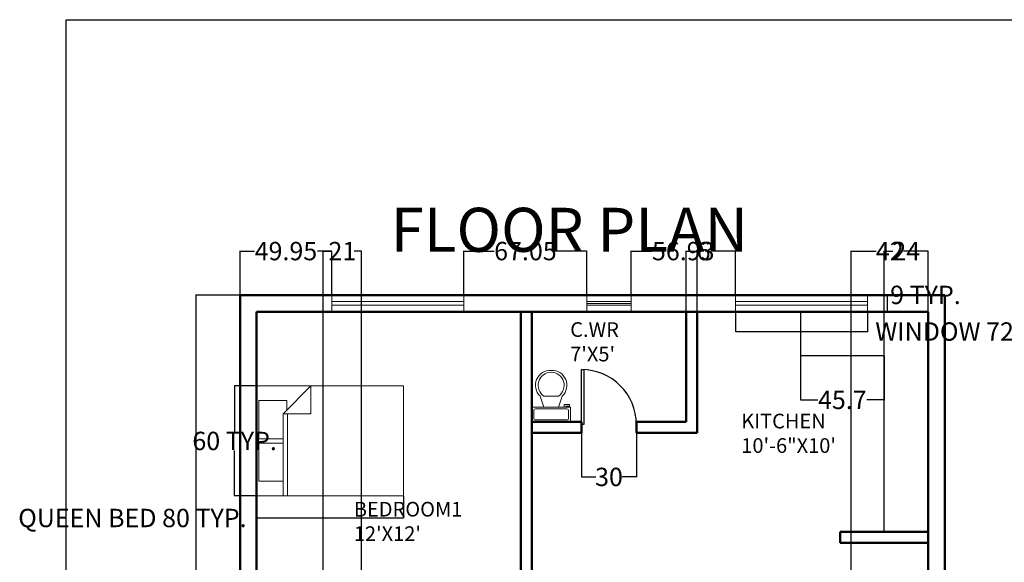
# Model space of a CAD drawing. Units: inches. Extents: x -16 to 1298, y 3 to 744.
# Tile 3 of 5: x -16 to 520, y 448 to 744. Entities that reach past the tile are written whole.
import ezdxf

# ---------------------------------------------------------------- set-up
doc = ezdxf.new("R2010")
doc.units = ezdxf.units.IN
doc.header["$MEASUREMENT"] = 0
for name, color, linetype, lineweight in [('A-ANNO-DIMS', 2, 'Continuous', 18), ('A-ANNO-TITL', 7, 'Continuous', 35), ('A-AREA-IDEN', 7, 'Continuous', 18), ('A-DOOR', 3, 'Continuous', 25), ('A-FLOR-CASE', 8, 'Continuous', 25), ('A-FLOR-FIXT', 9, 'Continuous', 18), ('A-FLOR-STRS', 7, 'Continuous', 25), ('A-FURN', 8, 'Continuous', 18), ('A-GLAZ', 4, 'Continuous', 18), ('A-WALL', 7, 'Continuous', 50)]:
    doc.layers.add(name, color=color, linetype=linetype, lineweight=lineweight)
doc.styles.get("Standard").update_dxf_attribs({"font": 'arial.ttf'})
doc.dimstyles.get("Standard").update_dxf_attribs({"dimtxt": 10, "dimasz": 0.18, "dimexe": 0.18, "dimexo": 0.0625, "dimgap": 0.09, "dimtad": 0, "dimtih": 1, "dimtoh": 1, "dimdec": 0, "dimzin": 0, "dimdsep": 46, "dimlunit": 3, "dimtxsty": 'Standard', "dimcen": 0.09, "dimadec": 0, "dimazin": 0, "dimtfac": 1, "dimtdec": 0, "dimtofl": 0, "dimtmove": 0, "dimatfit": 3, "dimfxl": 1, "dimtolj": 1, "dimtzin": 0, "dimarcsym": 0})

# ---------------------------------------------------------------- blocks, each defined once
blk = doc.blocks.new('Bed - Queen')
for p, q in [((0, -80.00003), (0, 0)), ((0, 0), (59.99999, 0)), ((59.99999, 0), (59.99999, -80.00003)), ((7.99999, -1.2), (28.79998, -1.2)), ((7.99999, -14.4), (7.99999, -1.2)), ((28.79998, -1.2), (28.79998, -14.4)), ((31.19999, -1.2), (51.99999, -1.2)), ((31.19999, -14.4), (31.19999, -1.2)), ((51.99999, -1.2), (51.99999, -16.4)), ((0, -14.4), (44.8, -14.4)), ((59.99999, -29.6), (44.8, -14.4)), ((44.8, -14.4), (44.8, -29.6)), ((44.8, -16.8), (0, -16.8)), ((51.99999, -16.4), (46.79936, -16.4)), ((44.8, -29.6), (59.99999, -29.6)), ((59.99999, -80.00003), (0, -80.00003))]:
    blk.add_line(p, q)
blk = doc.blocks.new('*U9')
for p, q in [((0, 0), (0, -6)), ((40, 0), (40, -6))]:
    blk.add_line(p, q)
blk.add_lwpolyline([(0, 0), (0, 40), (1.75, 40), (1.75, 0)], close=True)
blk.add_arc((0, 0), 40, 0, 90)
blk = doc.blocks.new('*U3')
for p, q in [((9.5, -6), (9.5, -2)), ((-10, -8.5), (-8, -8.5)), ((-10, -9.5), (-10, -8.5)), ((-7, -9.5), (-10, -9.5)), ((-8, -8.5), (-8, -8)), ((-7, -8), (-7, -9.5)), ((-4, -8), (-6, -14)), ((4, -8), (6, -14)), ((4, -14), (-4, -14))]:
    blk.add_line(p, q)
blk.add_lwpolyline([(10.5, -8), (10.5, 0), (-10.5, 0), (-10.5, -8)], close=True)
for points in [[(-9.5, -2), (-9.5, -6)], [(8.5, -1), (-8.5, -1)], [(-8.5, -7), (8.5, -7)]]:
    blk.add_lwpolyline(points)
for centre, radius, start, end in [((-8.625, -1.875), 0.8839, 81.8699, 188.1301), ((8.625, -1.875), 0.8839, 351.8699, 98.1301), ((-8.625, -6.125), 0.8839, 171.869898, 278.1301), ((8.625, -6.125), 0.8839, 261.8699, 8.1301), ((-0.4772, -19.9188), 8.0953, 133.01722, 273.38), ((0.0374, -19.8731), 7.127, 124.50543, 269.7), ((-0.0373, -19.8731), 7.127, 270.3, 55.4946), ((0.4773, -19.9188), 8.0953, 266.62, 46.9828)]:
    blk.add_arc(centre, radius, start, end)
blk = doc.blocks.new('WIN-72-WALL-9')
for p, q in [((0, 0), (0, 9)), ((72, 5.5), (0, 5.5)), ((72, 0), (72, 9)), ((72, 3.5), (0, 3.5))]:
    blk.add_line(p, q)
blk = doc.blocks.new('VENT-24-WALL-9')
for p, q in [((0, 0), (0, 9)), ((0, 5.5), (24, 5.5)), ((24, 0), (24, 9)), ((0, 4.5), (24, 4.5)), ((0, 3.5), (24, 3.5))]:
    blk.add_line(p, q)
blk = doc.blocks.new('*D26')
at = {"layer": 'A-ANNO-DIMS', "color": 0, "lineweight": -2, "transparency": 16777216}
for p, q in [((373.61, 584.93), (373.61, 574.01)), ((445.61, 584.93), (445.61, 574.01)), ((373.79, 574.19), (445.43, 574.19)), ((445.61, 574.19), (445.79, 574.19))]:
    blk.add_line(p, q, dxfattribs=at)
at = {"layer": 'A-ANNO-DIMS', "color": 0, "transparency": 16777216}
for points in [[(373.79, 574.22), (373.79, 574.16), (373.61, 574.19)], [(445.43, 574.22), (445.43, 574.16), (445.61, 574.19)]]:
    blk.add_solid(points, dxfattribs=at)
at = {"layer": 'Defpoints', "color": 0, "transparency": 16777216}
for p in [(373.61, 584.99), (445.61, 584.99), (445.61, 574.19)]:
    blk.add_point(p, dxfattribs=at)
at = {"layer": 'A-ANNO-DIMS', "color": 0, "transparency": 16777216, "insert": (503.01, 574.19), "char_height": 10, "attachment_point": 5}
blk.add_mtext('\\A1;WINDOW 72 TYP.', dxfattribs=at)
blk = doc.blocks.new('*D27')
at = {"layer": 'A-ANNO-DIMS', "color": 0, "lineweight": -2, "transparency": 16777216}
for p, q in [((445.67, 593.99), (456.59, 593.99)), ((456.41, 593.99), (456.41, 594.17)), ((456.41, 594.17), (456.59, 594.17)), ((456.41, 585.17), (456.41, 593.81)), ((445.67, 584.99), (456.59, 584.99))]:
    blk.add_line(p, q, dxfattribs=at)
at = {"layer": 'A-ANNO-DIMS', "color": 0, "transparency": 16777216}
for points in [[(456.38, 593.81), (456.44, 593.81), (456.41, 593.99)], [(456.38, 585.17), (456.44, 585.17), (456.41, 584.99)]]:
    blk.add_solid(points, dxfattribs=at)
at = {"layer": 'Defpoints', "color": 0, "transparency": 16777216}
for p in [(445.61, 593.99), (456.41, 593.99), (445.61, 584.99)]:
    blk.add_point(p, dxfattribs=at)
at = {"layer": 'A-ANNO-DIMS', "color": 0, "transparency": 16777216, "insert": (477.13, 594.17), "char_height": 10, "attachment_point": 5}
blk.add_mtext('\\A1;9 TYP.', dxfattribs=at)
blk = doc.blocks.new('*D30')
at = {"layer": 'A-ANNO-DIMS', "color": 0, "lineweight": -2, "transparency": 16777216}
for p, q in [((112.68, 484.49), (112.68, 472.37)), ((192.68, 484.49), (192.68, 472.37)), ((112.68, 472.55), (112.5, 472.55)), ((192.5, 472.55), (112.86, 472.55))]:
    blk.add_line(p, q, dxfattribs=at)
at = {"layer": 'A-ANNO-DIMS', "color": 0, "transparency": 16777216}
for points in [[(112.86, 472.58), (112.86, 472.52), (112.68, 472.55)], [(192.5, 472.58), (192.5, 472.52), (192.68, 472.55)]]:
    blk.add_solid(points, dxfattribs=at)
at = {"layer": 'Defpoints', "color": 0, "transparency": 16777216}
for p in [(112.68, 484.55), (192.68, 484.55), (112.68, 472.55)]:
    blk.add_point(p, dxfattribs=at)
at = {"layer": 'A-ANNO-DIMS', "color": 0, "transparency": 16777216, "insert": (45, 472.55), "char_height": 10, "attachment_point": 5}
blk.add_mtext('\\A1;QUEEN BED 80 TYP.', dxfattribs=at)
blk = doc.blocks.new('*D31')
at = {"layer": 'A-ANNO-DIMS', "color": 0, "lineweight": -2, "transparency": 16777216}
for p, q in [((112.61, 544.55), (100.5, 544.55)), ((100.68, 544.37), (100.68, 519.74)), ((100.68, 484.73), (100.68, 509.35)), ((112.61, 484.55), (100.5, 484.55))]:
    blk.add_line(p, q, dxfattribs=at)
at = {"layer": 'A-ANNO-DIMS', "color": 0, "transparency": 16777216}
for points in [[(100.65, 544.37), (100.71, 544.37), (100.68, 544.55)], [(100.65, 484.73), (100.71, 484.73), (100.68, 484.55)]]:
    blk.add_solid(points, dxfattribs=at)
at = {"layer": 'Defpoints', "color": 0, "transparency": 16777216}
for p in [(100.68, 544.55), (112.68, 544.55), (112.68, 484.55)]:
    blk.add_point(p, dxfattribs=at)
at = {"layer": 'A-ANNO-DIMS', "color": 0, "transparency": 16777216, "insert": (100.68, 514.55), "char_height": 10, "attachment_point": 5}
blk.add_mtext('\\A1;60 TYP.', dxfattribs=at)
blk = doc.blocks.new('*D41')
at = {"layer": 'A-ANNO-DIMS', "color": 0, "lineweight": -2, "transparency": 16777216}
for p, q in [((103.61, 593.99), (79.45, 593.99)), ((79.63, 593.81), (79.63, 383.19)), ((79.63, 162.17), (79.63, 372.79)), ((103.61, 161.99), (79.45, 161.99))]:
    blk.add_line(p, q, dxfattribs=at)
at = {"layer": 'A-ANNO-DIMS', "color": 0, "transparency": 16777216}
for points in [[(79.6, 593.81), (79.66, 593.81), (79.63, 593.99)], [(79.6, 162.17), (79.66, 162.17), (79.63, 161.99)]]:
    blk.add_solid(points, dxfattribs=at)
at = {"layer": 'Defpoints', "color": 0, "transparency": 16777216}
for p in [(79.63, 593.99), (103.68, 593.99), (103.68, 161.99)]:
    blk.add_point(p, dxfattribs=at)
at = {"layer": 'A-ANNO-DIMS', "color": 0, "transparency": 16777216, "insert": (79.63, 377.99), "char_height": 10, "attachment_point": 5}
blk.add_mtext('\\A1;432', dxfattribs=at)
blk = doc.blocks.new('*D42')
at = {"layer": 'A-ANNO-DIMS', "color": 0, "lineweight": -2, "transparency": 16777216}
for p, q in [((436.68, 237.05), (436.68, 618.22)), ((436.86, 618.04), (450.27, 618.04)), ((478.5, 618.04), (465.08, 618.04)), ((478.68, 237.05), (478.68, 618.22))]:
    blk.add_line(p, q, dxfattribs=at)
at = {"layer": 'A-ANNO-DIMS', "color": 0, "transparency": 16777216}
for points in [[(436.86, 618.07), (436.86, 618.01), (436.68, 618.04)], [(478.5, 618.07), (478.5, 618.01), (478.68, 618.04)]]:
    blk.add_solid(points, dxfattribs=at)
at = {"layer": 'Defpoints', "color": 0, "transparency": 16777216}
for p in [(478.68, 618.04), (436.68, 236.99), (478.68, 236.99)]:
    blk.add_point(p, dxfattribs=at)
at = {"layer": 'A-ANNO-DIMS', "color": 0, "transparency": 16777216, "insert": (457.68, 618.04), "char_height": 10, "attachment_point": 5}
blk.add_mtext('\\A1;42', dxfattribs=at)
blk = doc.blocks.new('*D45')
at = {"layer": 'A-ANNO-DIMS', "color": 0, "lineweight": -2, "transparency": 16777216}
for p, q in [((103.68, 594.05), (103.68, 618.22)), ((103.86, 618.04), (111.45, 618.04)), ((153.44, 618.04), (145.85, 618.04)), ((153.62, 594.05), (153.62, 618.22))]:
    blk.add_line(p, q, dxfattribs=at)
at = {"layer": 'A-ANNO-DIMS', "color": 0, "transparency": 16777216}
for points in [[(103.86, 618.07), (103.86, 618.01), (103.68, 618.04)], [(153.44, 618.07), (153.44, 618.01), (153.62, 618.04)]]:
    blk.add_solid(points, dxfattribs=at)
at = {"layer": 'Defpoints', "color": 0, "transparency": 16777216}
for p in [(153.62, 618.04), (103.68, 593.99), (153.62, 593.99)]:
    blk.add_point(p, dxfattribs=at)
at = {"layer": 'A-ANNO-DIMS', "color": 0, "transparency": 16777216, "insert": (128.65, 618.04), "char_height": 10, "attachment_point": 5}
blk.add_mtext('\\A1;49.95', dxfattribs=at)
blk = doc.blocks.new('*D46')
at = {"layer": 'A-ANNO-DIMS', "color": 0, "lineweight": -2, "transparency": 16777216}
for p, q in [((225.62, 594.05), (225.62, 618.22)), ((225.8, 618.04), (242.12, 618.04)), ((292.5, 618.04), (276.18, 618.04)), ((292.68, 594.05), (292.68, 618.22))]:
    blk.add_line(p, q, dxfattribs=at)
at = {"layer": 'A-ANNO-DIMS', "color": 0, "transparency": 16777216}
for points in [[(225.8, 618.07), (225.8, 618.01), (225.62, 618.04)], [(292.5, 618.07), (292.5, 618.01), (292.68, 618.04)]]:
    blk.add_solid(points, dxfattribs=at)
at = {"layer": 'Defpoints', "color": 0, "transparency": 16777216}
for p in [(292.68, 618.04), (225.62, 593.99), (292.68, 593.99)]:
    blk.add_point(p, dxfattribs=at)
at = {"layer": 'A-ANNO-DIMS', "color": 0, "transparency": 16777216, "insert": (259.15, 618.04), "char_height": 10, "attachment_point": 5}
blk.add_mtext('\\A1;67.05', dxfattribs=at)
blk = doc.blocks.new('*D47')
at = {"layer": 'A-ANNO-DIMS', "color": 0, "lineweight": -2, "transparency": 16777216}
for p, q in [((316.68, 594.05), (316.68, 618.22)), ((316.86, 618.04), (328.18, 618.04)), ((373.43, 618.04), (362.1, 618.04)), ((373.61, 594.05), (373.61, 618.22))]:
    blk.add_line(p, q, dxfattribs=at)
at = {"layer": 'A-ANNO-DIMS', "color": 0, "transparency": 16777216}
for points in [[(316.86, 618.07), (316.86, 618.01), (316.68, 618.04)], [(373.43, 618.07), (373.43, 618.01), (373.61, 618.04)]]:
    blk.add_solid(points, dxfattribs=at)
at = {"layer": 'Defpoints', "color": 0, "transparency": 16777216}
for p in [(373.61, 618.04), (316.68, 593.99), (373.61, 593.99)]:
    blk.add_point(p, dxfattribs=at)
at = {"layer": 'A-ANNO-DIMS', "color": 0, "transparency": 16777216, "insert": (345.14, 618.04), "char_height": 10, "attachment_point": 5}
blk.add_mtext('\\A1;56.93', dxfattribs=at)
blk = doc.blocks.new('*D55')
at = {"layer": 'A-ANNO-DIMS', "color": 0, "lineweight": -2, "transparency": 16777216}
for p, q in [((289.68, 518.93), (289.68, 494.76)), ((319.68, 518.93), (319.68, 494.76)), ((289.86, 494.94), (297.44, 494.94)), ((319.5, 494.94), (311.91, 494.94))]:
    blk.add_line(p, q, dxfattribs=at)
at = {"layer": 'A-ANNO-DIMS', "color": 0, "transparency": 16777216}
for points in [[(289.86, 494.97), (289.86, 494.91), (289.68, 494.94)], [(319.5, 494.97), (319.5, 494.91), (319.68, 494.94)]]:
    blk.add_solid(points, dxfattribs=at)
at = {"layer": 'Defpoints', "color": 0, "transparency": 16777216}
for p in [(289.68, 518.99), (319.68, 518.99), (289.68, 494.94)]:
    blk.add_point(p, dxfattribs=at)
at = {"layer": 'A-ANNO-DIMS', "color": 0, "transparency": 16777216, "insert": (304.68, 494.94), "char_height": 10, "attachment_point": 5}
blk.add_mtext('\\A1;30', dxfattribs=at)
blk = doc.blocks.new('*D56')
at = {"layer": 'A-ANNO-DIMS', "color": 0, "lineweight": -2, "transparency": 16777216}
for p, q in [((346.68, 525.05), (346.68, 618.22)), ((346.86, 618.04), (352.5, 618.04)), ((352.68, 519.05), (352.68, 618.22)), ((352.68, 618.04), (352.86, 618.04))]:
    blk.add_line(p, q, dxfattribs=at)
at = {"layer": 'A-ANNO-DIMS', "color": 0, "transparency": 16777216}
for points in [[(346.86, 618.07), (346.86, 618.01), (346.68, 618.04)], [(352.5, 618.07), (352.5, 618.01), (352.68, 618.04)]]:
    blk.add_solid(points, dxfattribs=at)
at = {"layer": 'Defpoints', "color": 0, "transparency": 16777216}
for p in [(352.68, 618.04), (346.68, 524.99), (352.68, 518.99)]:
    blk.add_point(p, dxfattribs=at)
at = {"layer": 'A-ANNO-DIMS', "color": 0, "transparency": 16777216, "insert": (356.25, 618.04), "char_height": 10, "attachment_point": 5}
blk.add_mtext('\\A1;6', dxfattribs=at)
blk = doc.blocks.new('*D57')
at = {"layer": 'A-ANNO-DIMS', "color": 0, "lineweight": -2, "transparency": 16777216}
for p, q in [((454.68, 465.05), (454.68, 618.22)), ((454.86, 618.04), (459.36, 618.04)), ((478.5, 618.04), (473.99, 618.04)), ((478.68, 465.05), (478.68, 618.22))]:
    blk.add_line(p, q, dxfattribs=at)
at = {"layer": 'A-ANNO-DIMS', "color": 0, "transparency": 16777216}
for points in [[(454.86, 618.07), (454.86, 618.01), (454.68, 618.04)], [(478.5, 618.07), (478.5, 618.01), (478.68, 618.04)]]:
    blk.add_solid(points, dxfattribs=at)
at = {"layer": 'Defpoints', "color": 0, "transparency": 16777216}
for p in [(478.68, 618.04), (454.68, 464.99), (478.68, 464.99)]:
    blk.add_point(p, dxfattribs=at)
at = {"layer": 'A-ANNO-DIMS', "color": 0, "transparency": 16777216, "insert": (466.68, 618.04), "char_height": 10, "attachment_point": 5}
blk.add_mtext('\\A1;24', dxfattribs=at)
blk = doc.blocks.new('*D58')
at = {"layer": 'A-ANNO-DIMS', "color": 0, "lineweight": -2, "transparency": 16777216}
for p, q in [((408.98, 560.93), (408.98, 536.76)), ((454.68, 560.93), (454.68, 536.76)), ((409.16, 536.94), (418.55, 536.94)), ((454.5, 536.94), (445.11, 536.94))]:
    blk.add_line(p, q, dxfattribs=at)
at = {"layer": 'A-ANNO-DIMS', "color": 0, "transparency": 16777216}
for points in [[(409.16, 536.97), (409.16, 536.91), (408.98, 536.94)], [(454.5, 536.97), (454.5, 536.91), (454.68, 536.94)]]:
    blk.add_solid(points, dxfattribs=at)
at = {"layer": 'Defpoints', "color": 0, "transparency": 16777216}
for p in [(408.98, 560.99), (454.68, 560.99), (408.98, 536.94)]:
    blk.add_point(p, dxfattribs=at)
at = {"layer": 'A-ANNO-DIMS', "color": 0, "transparency": 16777216, "insert": (431.83, 536.94), "char_height": 10, "attachment_point": 5}
blk.add_mtext('\\A1;45.7', dxfattribs=at)
blk = doc.blocks.new('*D61')
at = {"layer": 'A-ANNO-DIMS', "color": 0, "lineweight": -2, "transparency": 16777216}
for p, q in [((148.9, 375.05), (148.9, 618.22)), ((149.08, 618.04), (153.03, 618.04)), ((169.72, 618.04), (165.77, 618.04)), ((169.9, 375.05), (169.9, 618.22))]:
    blk.add_line(p, q, dxfattribs=at)
at = {"layer": 'A-ANNO-DIMS', "color": 0, "transparency": 16777216}
for points in [[(149.08, 618.07), (149.08, 618.01), (148.9, 618.04)], [(169.72, 618.07), (169.72, 618.01), (169.9, 618.04)]]:
    blk.add_solid(points, dxfattribs=at)
at = {"layer": 'Defpoints', "color": 0, "transparency": 16777216}
for p in [(169.9, 618.04), (148.9, 374.99), (169.9, 374.99)]:
    blk.add_point(p, dxfattribs=at)
at = {"layer": 'A-ANNO-DIMS', "color": 0, "transparency": 16777216, "insert": (159.4, 618.04), "char_height": 10, "attachment_point": 5}
blk.add_mtext('\\A1;21', dxfattribs=at)

msp = doc.modelspace()

# ---------------------------------------------------------------- linework, layer by layer
at = {"layer": 'A-FLOR-CASE'}
for p, q in [((408.9777, 584.9884), (408.9777, 560.9884)), ((454.6768, 560.9884), (408.9777, 560.9884)), ((454.6768, 464.9884), (454.6768, 560.9884))]:
    msp.add_line(p, q, dxfattribs=at)
at = {"layer": 'A-FLOR-STRS'}
msp.add_line((436.6768, 416.9884), (436.6768, 458.9884), dxfattribs=at)
at = {"layer": 'A-WALL'}
for p, q in [((487.6768, 593.9884), (103.6768, 593.9884)), ((103.6768, 593.9884), (103.6768, 161.9884)), ((487.6768, 161.9884), (487.6768, 593.9884)), ((478.6768, 584.9884), (112.6768, 584.9884)), ((112.6768, 584.9884), (112.6768, 170.9884)), ((256.6768, 584.9884), (256.6768, 412.9884)), ((262.6768, 584.9884), (262.6768, 412.9884)), ((262.6768, 584.9884), (346.6768, 584.9884)), ((346.6768, 584.9884), (346.6768, 524.9884)), ((352.6768, 584.9884), (352.6768, 518.9884)), ((478.6768, 161.9884), (478.6768, 584.9884)), ((262.6768, 524.9884), (289.6768, 524.9884)), ((289.6768, 524.9884), (262.6768, 524.9884)), ((289.6768, 524.9884), (289.6768, 518.9884)), ((346.6768, 524.9884), (319.6768, 524.9884)), ((319.6768, 524.9884), (319.6768, 518.9884)), ((319.6768, 524.9884), (346.6768, 524.9884)), ((289.6768, 518.9884), (262.6768, 518.9884)), ((352.6768, 518.9884), (319.6768, 518.9884)), ((478.6768, 464.9884), (430.6768, 464.9884)), ((430.6768, 464.9884), (430.6768, 458.9884)), ((478.6768, 458.9884), (430.6768, 458.9884))]:
    msp.add_line(p, q, dxfattribs=at)
at = {"layer": 'Defpoints'}
msp.add_lwpolyline([(8.9336, 744.17), (1298.346, 744.17), (1298.346, 3.4476), (8.9336, 3.4476)], close=True, dxfattribs=at)

# ---------------------------------------------------------------- block references
at = {"layer": 'A-DOOR', "xscale": 0.7490164830143604, "yscale": 0.7490164830143604, "zscale": 0.7490164830143604}
msp.add_blockref('*U9', (289.6768, 523.4825), dxfattribs=at)
at = {"layer": 'A-FLOR-FIXT', "rotation": 180}
msp.add_blockref('*U3', (273.1768, 524.9884), dxfattribs=at)
at = {"layer": 'A-FURN', "rotation": 90}
msp.add_blockref('Bed - Queen', (112.6768, 484.5483), dxfattribs=at)
at = {"layer": 'A-GLAZ'}
for name, p in [('WIN-72-WALL-9', (153.6224, 584.9884)), ('VENT-24-WALL-9', (292.6768, 584.9884)), ('WIN-72-WALL-9', (373.6051, 584.9884))]:
    msp.add_blockref(name, p, dxfattribs=at)

# ---------------------------------------------------------------- texts
at = {"layer": 'A-ANNO-TITL', "insert": (185.7307, 641.6404), "char_height": 24, "attachment_point": 1}
msp.add_mtext_dynamic_manual_height_columns('{\\fTimes New Roman|b0|i0|c0|p18;FLOOR PLAN}', width=347.060427, gutter_width=1, heights=[0], dxfattribs=at)
at = {"layer": 'A-AREA-IDEN', "char_height": 8, "attachment_point": 1}
for s, heights, insert in [("C.WR\\P7'X5'", [0], (283.5532, 579.2675)), ('KITCHEN\\P10\'-6"X10\'', [0], (376.7752, 529.388)), ("BEDROOM1\\P12'X12'", [34.8911], (165.6491, 481.3444))]:
    msp.add_mtext_dynamic_manual_height_columns(s, width=63.245227, gutter_width=1, heights=heights, dxfattribs=dict(at, insert=insert))

# ---------------------------------------------------------------- dimensions: what is measured, and where the dimension line sits
at = {"layer": 'A-ANNO-DIMS'}
for base, p1, p2, override, picture, middle in [((153.6224, 618.0384), (103.6768, 593.9884), (153.6224, 593.9884), {"dimdec": 2, "dimlfac": 1, "dimrnd": 0, "dimzin": 0, "dimdsep": 46, "dimlunit": 2}, '*D45', (128.6496, 618.0384)), ((169.8975, 618.0384), (148.8975, 374.9884), (169.8975, 374.9884), {"dimdec": 0, "dimlfac": 1, "dimrnd": 0, "dimzin": 0, "dimdsep": 46, "dimlunit": 2}, '*D61', (159.3975, 618.0384)), ((292.6768, 618.0384), (225.6224, 593.9884), (292.6768, 593.9884), {"dimdec": 2, "dimlfac": 1, "dimrnd": 0, "dimzin": 0, "dimdsep": 46, "dimlunit": 2}, '*D46', (259.1496, 618.0384)), ((373.6051, 618.0384), (316.6768, 593.9884), (373.6051, 593.9884), {"dimdec": 2, "dimlfac": 1, "dimrnd": 0, "dimzin": 0, "dimdsep": 46, "dimlunit": 2}, '*D47', (345.141, 618.0384)), ((352.6768, 618.0384), (346.6768, 524.9884), (352.6768, 518.9884), {"dimdec": 0, "dimlfac": 1, "dimrnd": 0, "dimzin": 0, "dimdsep": 46, "dimlunit": 2}, '*D56', (356.2483, 618.0384)), ((478.6768, 618.0384), (436.6768, 236.9884), (478.6768, 236.9884), {"dimdec": 0, "dimlfac": 1, "dimrnd": 0, "dimzin": 0, "dimdsep": 46, "dimlunit": 2}, '*D42', (457.6768, 618.0384)), ((478.6768, 618.0384), (454.6768, 464.9884), (478.6768, 464.9884), {"dimdec": 0, "dimlfac": 1, "dimrnd": 0, "dimzin": 0, "dimdsep": 46, "dimlunit": 2}, '*D57', (466.6768, 618.0384))]:
    dim = msp.add_linear_dim(base=base, p1=p1, p2=p2, dimstyle='Standard', override=override, dxfattribs=at)
    dim.commit()
    dim.dimension.update_dxf_attribs({"geometry": picture, "text_midpoint": middle})
for base, p1, p2, angle, text, picture, middle in [((456.4051, 593.9884), (445.6051, 584.9884), (445.6051, 593.9884), 90, '<> TYP.', '*D27', (477.1288, 594.1684)), ((100.6768, 544.5483), (112.6768, 484.5483), (112.6768, 544.5483), 90, '<> TYP.', '*D31', (100.6768, 514.5483)), ((112.6768, 472.5483), (192.6768, 484.5483), (112.6768, 484.5483), 180, 'QUEEN BED <> TYP.', '*D30', (44.9955, 472.5483))]:
    dim = msp.add_linear_dim(base=base, p1=p1, p2=p2, angle=angle, text=text, dimstyle='Standard', override={"dimdec": 0, "dimlfac": 1, "dimrnd": 0, "dimzin": 0, "dimdsep": 46, "dimlunit": 2}, dxfattribs=at)
    dim.commit()
    dim.dimension.update_dxf_attribs({"geometry": picture, "text_midpoint": middle})
dim = msp.add_linear_dim(base=(445.6051, 574.1884), p1=(373.6051, 584.9884), p2=(445.6051, 584.9884), text='WINDOW <> TYP.', dimstyle='Standard', override={"dimdec": 0, "dimlfac": 1, "dimrnd": 0, "dimzin": 0, "dimdsep": 46, "dimlunit": 2}, dxfattribs=at)
dim.commit()
dim.dimension.update_dxf_attribs({"geometry": '*D26', "text_midpoint": (503.0068, 574.1884)})
for base, p1, p2, angle, override, picture, middle in [((79.6268, 593.9884), (103.6768, 161.9884), (103.6768, 593.9884), 90, {"dimdec": 0, "dimlfac": 1, "dimrnd": 0, "dimzin": 0, "dimdsep": 46, "dimlunit": 2}, '*D41', (79.6268, 377.9884)), ((408.9777, 536.9384), (454.6768, 560.9884), (408.9777, 560.9884), 180, {"dimdec": 1, "dimlfac": 1, "dimrnd": 0, "dimzin": 0, "dimdsep": 46, "dimlunit": 2}, '*D58', (431.8272, 536.9384)), ((289.6768, 494.9384), (319.6768, 518.9884), (289.6768, 518.9884), 180, {"dimdec": 0, "dimlfac": 1, "dimrnd": 0, "dimzin": 0, "dimdsep": 46, "dimlunit": 2}, '*D55', (304.6768, 494.9384))]:
    dim = msp.add_linear_dim(base=base, p1=p1, p2=p2, angle=angle, dimstyle='Standard', override=override, dxfattribs=at)
    dim.commit()
    dim.dimension.update_dxf_attribs({"geometry": picture, "text_midpoint": middle})

doc.saveas('drawing.dxf')
